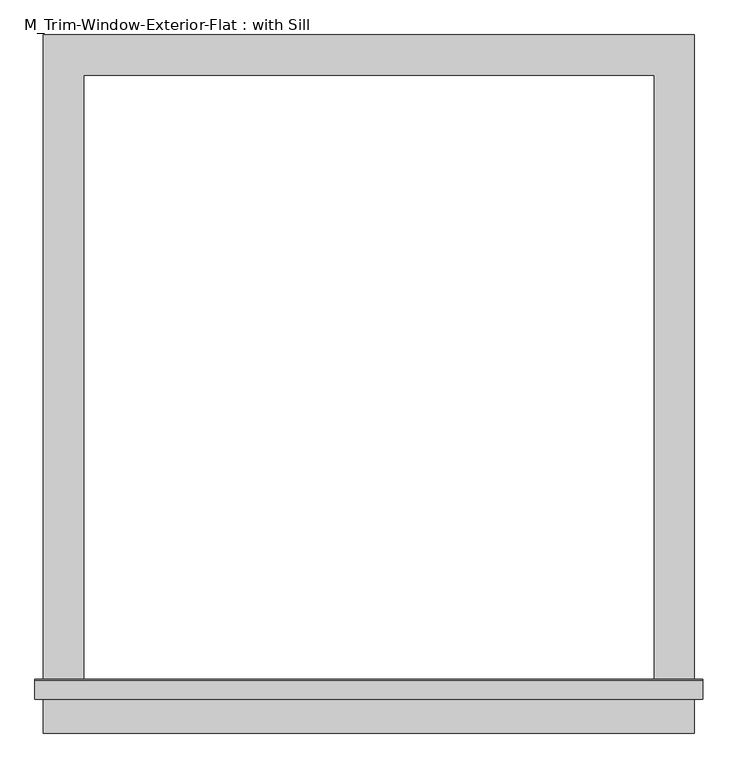
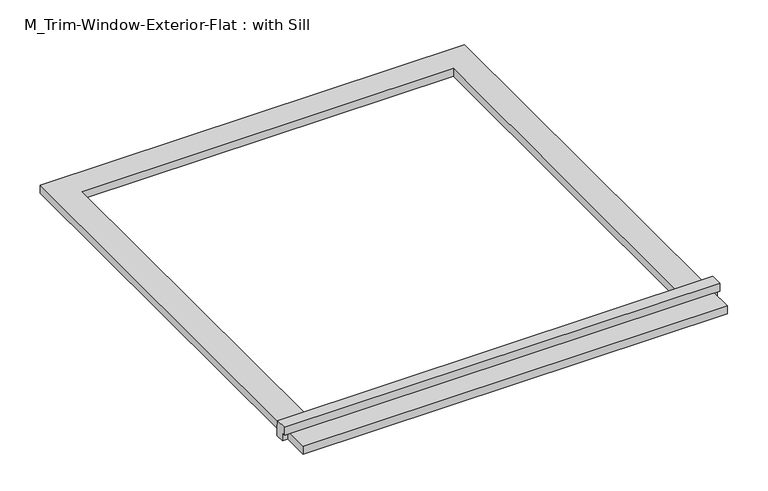
"""IFC4 building model written with IfcOpenShell, lengths in millimetres: proxy geometry, M_Trim-Window-Exterior-Flat : with Sill."""

from ifc_helpers import new_model, si_unit, frame, origin, origin_with_axes, place, context, project, spatial, polyline, outline, extrude, source, transform, mapped, element, save


def m_trim_window_exterior_flat_with_sill_90d3a428(model_context):
    return source(origin(), model_context, "Body", "SweptSolid", [
        extrude(outline(polyline([(485.0, -920.4323709), (485.0, -980.4323709), (-485.0, -980.4323709), (-485.0, -920.4323709), (485.0, -920.4323709)])), origin_with_axes(), (0.0, 0.0, 1.0), 19.05),
        extrude(outline(polyline([(-930.0, 38.1), (-902.4580645, 38.1), (-900.0, 19.05), (-900.0, 0.0), (-920.4323709, 0.0), (-920.4323709, 19.05), (-930.0, 19.05), (-930.0, 38.1)])), frame((-497.7, 0.0, 0.0), z_axis=(1.0, 0.0, 0.0), x_axis=(0.0, 1.0, 0.0)), (0.0, 0.0, 1.0), 995.4),
        extrude(outline(polyline([(-485.0, 60.0), (485.0, 60.0), (485.0, -900.0), (425.0, -900.0), (425.0, 0.0), (-425.0, 0.0), (-425.0, -900.0), (-485.0, -900.0), (-485.0, 60.0)])), origin_with_axes(), (0.0, 0.0, 1.0), 19.05),
    ])


if __name__ == "__main__":
    model = new_model("IFC4")
    model_context = context("Model", 3, world=origin())
    ifc_project = project(units=[si_unit("LENGTHUNIT", "METRE", prefix="MILLI")], contexts=[model_context])
    site = spatial("IfcSite", under=ifc_project)
    building = spatial("IfcBuilding", under=site)
    placement = place(None, origin())
    m_trim_window_exterior_flat_with_sill_shape = m_trim_window_exterior_flat_with_sill_90d3a428(model_context)
    element("IfcBuildingElementProxy", 1, Name="M_Trim-Window-Exterior-Flat : with Sill", ObjectType="M_Trim-Window-Exterior-Flat : with Sill", at=placement, inside=building, context=model_context, shape_type="MappedRepresentation", body=[
        mapped(m_trim_window_exterior_flat_with_sill_shape, transform((0.0, 0.0, 0.0), x_axis=(1.0, 0.0, 0.0), y_axis=(0.0, 1.0, 0.0), z_axis=(0.0, 0.0, 1.0))),
    ])
    save(model, "model.ifc")

# Revit data of these elements
# Type "M_Trim-Window-Exterior-Flat : with Sill"
#   Trim Width = 60 mm
#   Trim Thickness_Picture Frame = 30 mm
#   Trim Thickness_with Sill = 19.05 mm
#   Sill Thickness = 30 mm
#   Opening Width [instance default] = 600 mm
#   Opening Height [instance default] = 900 mm
#   Default Elevation = 1200 mm
#   Sill = yes
#   Picture Frame = no
#   Trim Material [instance default] = none
# Element 1 (IfcBuildingElementProxy, "M_Trim-Window-Exterior-Flat : with Sill")
#   Opening Width = 850 mm
#   Trim Material = Clad - White
#   Materials on its faces: "Clad - White"
# Materials
#   "Clad - White": class "Wood", colour RGB 242 242 238, transparency 0, Cost = 0
